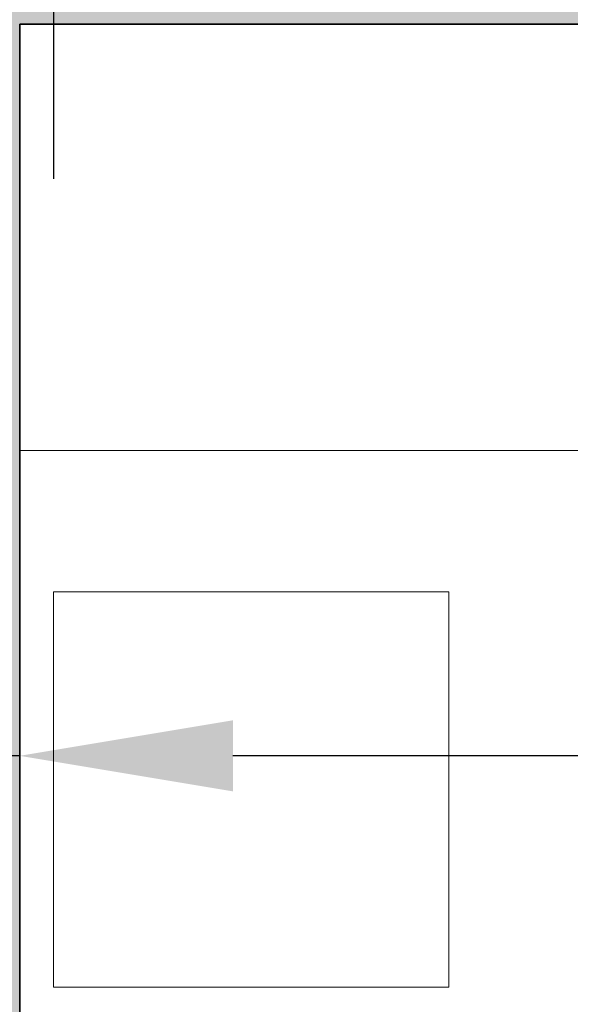
# Model space of a CAD drawing. Units: inches. Extents: x 2083 to 3317, y 1141 to 2115.
# Tile 12 of 256: x 2236 to 2267, y 1361 to 1417. Entities that reach past the tile are written whole.
import ezdxf

# ---------------------------------------------------------------- set-up
doc = ezdxf.new("R2010")
doc.units = ezdxf.units.IN
for name, color, linetype, lineweight in [('A-ANNO-DIMS', 2, 'Continuous', 18), ('A-FLOR-CASE', 8, 'Continuous', 18), ('A-FURN', 8, 'Continuous', 18), ('A-WALL', 7, 'Continuous', 35)]:
    doc.layers.add(name, color=color, linetype=linetype, lineweight=lineweight)
doc.layers.add('A-WALL-PATT', color=251, linetype='Continuous', lineweight=13, true_color=0x636466)
doc.styles.get("Standard").update_dxf_attribs({"font": 'arial.ttf'})
doc.dimstyles.new('ISO-25', dxfattribs={"dimtxt": 12, "dimasz": 12, "dimexe": 1.25, "dimexo": 0.625, "dimtad": 1, "dimlunit": 3, "dimtxsty": 'Standard', "dimcen": 2.5, "dimadec": 0, "dimazin": 0, "dimtfac": 1, "dimtmove": 0, "dimatfit": 3, "dimfxl": 1, "dimarcsym": 0})

# ---------------------------------------------------------------- blocks, each defined once
blk = doc.blocks.new('CASEWORK-96X24')
blk.add_line((0, 96), (0, 0))
blk = doc.blocks.new('NIGHTSTAND-COMPACT')
blk.add_lwpolyline([(22.254, 22.255), (22.254, 0), (0, 0), (0, 22.255)], close=True)
blk = doc.blocks.new('*D22')
at = {"layer": 'A-ANNO-DIMS', "color": 0, "lineweight": -2, "transparency": 16777216}
for p, q in [((2235.96, 1362.739), (2235.96, 1376.309)), ((2322.26, 1362.739), (2322.26, 1376.309)), ((2235.96, 1375.059), (2083.007, 1375.059)), ((2310.26, 1375.059), (2247.96, 1375.059))]:
    blk.add_line(p, q, dxfattribs=at)
at = {"layer": 'A-ANNO-DIMS', "color": 0, "transparency": 16777216}
for points in [[(2247.96, 1377.059), (2247.96, 1373.059), (2235.96, 1375.059)], [(2310.26, 1377.059), (2310.26, 1373.059), (2322.26, 1375.059)]]:
    blk.add_solid(points, dxfattribs=at)
at = {"layer": 'Defpoints', "color": 0, "transparency": 16777216}
for p in [(2235.96, 1375.059), (2235.96, 1362.114), (2322.26, 1362.114)]:
    blk.add_point(p, dxfattribs=at)
at = {"layer": 'A-ANNO-DIMS', "color": 0, "transparency": 16777216, "insert": (2153.483, 1381.889), "char_height": 12, "attachment_point": 5}
blk.add_mtext('BED 7\'-2 1/2" TYP.', dxfattribs=at)
blk = doc.blocks.new('*D30')
at = {"layer": 'A-ANNO-DIMS', "color": 0, "lineweight": -2, "transparency": 16777216}
for p, q in [((2240.018, 1445.274), (2240.018, 1448.046)), ((2254.329, 1445.274), (2254.329, 1448.046)), ((2228.018, 1446.796), (2216.018, 1446.796)), ((2240.018, 1446.796), (2254.329, 1446.796)), ((2266.329, 1446.796), (2413.765, 1446.796))]:
    blk.add_line(p, q, dxfattribs=at)
at = {"layer": 'A-ANNO-DIMS', "color": 0, "transparency": 16777216}
for points in [[(2228.018, 1448.796), (2228.018, 1444.796), (2240.018, 1446.796)], [(2266.329, 1448.796), (2266.329, 1444.796), (2254.329, 1446.796)]]:
    blk.add_solid(points, dxfattribs=at)
at = {"layer": 'Defpoints', "color": 0, "transparency": 16777216}
for p in [(2254.329, 1446.796), (2240.018, 1444.649), (2254.329, 1444.649)]:
    blk.add_point(p, dxfattribs=at)
at = {"layer": 'A-ANNO-DIMS', "color": 0, "transparency": 16777216, "insert": (2346.047, 1453.625), "char_height": 12, "attachment_point": 5}
blk.add_mtext('WC 1\'-2 1/2" TYP.', dxfattribs=at)
blk = doc.blocks.new('*D31')
at = {"layer": 'A-ANNO-DIMS', "color": 0, "lineweight": -2, "transparency": 16777216}
for p, q in [((2237.871, 1456.649), (2237.871, 1541.915)), ((2239.393, 1444.649), (2236.621, 1444.649)), ((2237.871, 1431.548), (2237.871, 1444.649)), ((2239.393, 1431.548), (2236.621, 1431.548)), ((2237.871, 1419.548), (2237.871, 1407.548))]:
    blk.add_line(p, q, dxfattribs=at)
at = {"layer": 'A-ANNO-DIMS', "color": 0, "transparency": 16777216}
for points in [[(2235.871, 1456.649), (2239.871, 1456.649), (2237.871, 1444.649)], [(2235.871, 1419.548), (2239.871, 1419.548), (2237.871, 1431.548)]]:
    blk.add_solid(points, dxfattribs=at)
at = {"layer": 'Defpoints', "color": 0, "transparency": 16777216}
for p in [(2237.871, 1444.649), (2240.018, 1444.649), (2240.018, 1431.548)]:
    blk.add_point(p, dxfattribs=at)
at = {"layer": 'A-ANNO-DIMS', "color": 0, "transparency": 16777216, "insert": (2231.217, 1505.282), "char_height": 12, "attachment_point": 5, "rotation": 90}
blk.add_mtext('1\'-1" TYP.', dxfattribs=at)

msp = doc.modelspace()

# ---------------------------------------------------------------- hatches: boundary and pattern name
at = {"layer": 'A-WALL-PATT'}
h = msp.add_hatch(color=256, dxfattribs=at)
h.dxf.hatch_style = 1
h.paths.add_polyline_path([(3126.96, 2020.761), (2748.96, 2020.761), (2604.96, 2020.761), (2226.96, 2020.761), (2226.96, 1702.761), (2466.96, 1702.761), (2466.96, 1582.761), (2418.96, 1582.761), (2418.96, 1477.761), (2226.96, 1477.761), (2226.96, 1263.261), (2544.96, 1263.261), (2544.96, 1411.761), (2604.96, 1411.761), (2685.96, 1411.761), (2685.96, 1420.761), (2604.96, 1420.761), (2604.96, 1573.761), (2604.96, 1702.761), (2604.96, 2011.761), (2748.96, 2011.761), (2748.96, 1702.761), (2862.96, 1702.761), (2862.96, 1621.761), (2871.96, 1621.761), (2871.96, 1702.761), (2883.96, 1702.761), (2883.96, 1706.939, -0.026459), (2883.96, 1711.761), (2757.96, 1711.761), (2757.96, 1807.761), (2787.96, 1807.761), (2787.96, 1812.261), (2757.96, 1812.261), (2757.96, 2011.761), (2877.96, 2011.761), (2877.96, 1812.261), (2847.96, 1812.261), (2847.96, 1807.761), (2889.836, 1807.761), (2889.836, 1812.261), (2882.46, 1812.261), (2882.46, 2011.761), (3117.96, 2011.761), (3117.96, 1812.261), (2937.836, 1812.261), (2937.836, 1807.761), (2995.71, 1807.761), (2995.71, 1796.118), (3000.21, 1796.118), (3000.21, 1807.761), (3117.96, 1807.761), (3117.96, 1711.761), (3000.21, 1711.761), (3000.21, 1760.118), (2998.573, 1760.118, -0.020711), (2995.71, 1760.118), (2995.71, 1711.761), (2931.96, 1711.761), (2931.96, 1702.761), (3126.96, 1702.761)])
h.paths.add_polyline_path([(2471.46, 2011.761), (2471.46, 1810.011), (2462.717, 1810.011), (2462.717, 1805.511), (2505.96, 1805.511), (2505.96, 1810.011), (2475.96, 1810.011), (2475.96, 2011.761), (2595.96, 2011.761), (2595.96, 1810.011), (2565.96, 1810.011), (2565.96, 1805.511), (2595.96, 1805.511), (2595.96, 1711.761), (2235.96, 1711.761), (2235.96, 1805.511), (2353.71, 1805.511), (2353.71, 1796.054), (2358.21, 1796.054), (2358.21, 1805.511), (2414.717, 1805.511), (2414.717, 1810.011), (2235.96, 1810.011), (2235.96, 2011.761)], flags=16)
h.paths.add_polyline_path([(2270.205, 1994.61), (2270.205, 1970.61), (2246.205, 1970.61), (2246.205, 1994.61)], flags=0)
edge = h.paths.add_edge_path(flags=0)
edge.add_ellipse((2332.027, 1899.798), major_axis=(-3.043, 3.043), ratio=0.168252, start_angle=-161.3322, end_angle=-156.3071, ccw=False)
edge.add_ellipse((2333.082, 1898.744), major_axis=(-1.055, 1.055), ratio=0.453532, start_angle=-123.371, end_angle=-94.1591)
edge = h.paths.add_edge_path(flags=0)
edge.add_ellipse((2332.027, 1968.876), major_axis=(3.043, 3.043), ratio=0.168252, start_angle=18.6678, end_angle=23.6929)
edge.add_spline(control_points=[(2332.926, 1970.691), (2332.227, 1970.336), (2330.894, 1969.659), (2328.413, 1970.932), (2327.204, 1967.749), (2324.71, 1969.956), (2322.533, 1967.012), (2320.013, 1971.296), (2317.68, 1968.158), (2316.041, 1967.102), (2315.427, 1966.81)], knot_values=[0, 0, 0, 0, 2.267059, 4.324559, 6.685584, 8.878641, 11.121502, 14.300359, 17.755284, 19.732645, 19.732645, 19.732645, 19.732645], degree=3, periodic=0)
edge.add_ellipse((2332.027, 1968.876), major_axis=(3.043, 3.043), ratio=0.168252, start_angle=18.6678, end_angle=23.6929, ccw=False)
edge.add_ellipse((2333.082, 1969.931), major_axis=(1.055, 1.055), ratio=0.453532, start_angle=56.629, end_angle=85.8409, ccw=False)
edge = h.paths.add_edge_path(flags=0)
edge.add_spline(control_points=[(2296.428, 1967.988), (2293.628, 1965.336), (2287.704, 1959.727), (2299.744, 1949.996), (2294.533, 1935.669), (2290.573, 1920.604), (2293.394, 1909.974), (2296.185, 1904.967)], knot_values=[0.099185, 0.099185, 0.099185, 0.099185, 0.345301, 0.619822, 0.982653, 1.386093, 1.810555, 1.810555, 1.810555, 1.810555], degree=3, periodic=0)
edge.add_spline(control_points=[(2296.185, 1904.967), (2297.384, 1902.619), (2298.001, 1901.949), (2298.553, 1901.468)], knot_values=[0.006246, 0.006246, 0.006246, 0.006246, 0.055476, 0.055476, 0.055476, 0.055476], degree=3, periodic=0)
edge.add_spline(control_points=[(2298.553, 1901.468), (2297.259, 1900.923), (2295.225, 1900.232), (2293.06, 1900.614), (2292.101, 1900.788), (2292.09, 1900.791)], knot_values=[0.312835, 0.312835, 0.312835, 0.312835, 0.40178, 0.474987, 0.475903, 0.475903, 0.475903, 0.475903], degree=3, periodic=0)
edge.add_arc((2292.794, 1904.664), 3.937, 215.4209, 259.6982, ccw=False)
edge.add_spline(control_points=[(2289.585, 1902.382), (2289.477, 1902.535), (2289.368, 1902.688), (2289.261, 1902.841)], knot_values=[0.102872, 0.102872, 0.102872, 0.102872, 0.116896, 0.116896, 0.116896, 0.116896], degree=3, periodic=0)
edge.add_spline(control_points=[(2289.261, 1902.841), (2288.687, 1902.55), (2287.64, 1902.02), (2285.881, 1901.874), (2283.853, 1901.504), (2281.72, 1899.711), (2278.467, 1899.493), (2276.157, 1901.883), (2272.259, 1899.804), (2267.778, 1901.843), (2262.244, 1900.184), (2257.415, 1901.782), (2254.318, 1900.726), (2253.178, 1900.337)], knot_values=[0, 0, 0, 0, 1.907977, 3.477176, 5.261074, 7.972851, 11.680248, 13.717921, 16.939592, 22.789562, 27.502503, 33.595215, 37.145618, 37.145618, 37.145618, 37.145618], degree=3, periodic=0)
edge.add_line((2253.178, 1900.337), (2250.244, 1902.841))
edge.add_line((2250.244, 1902.841), (2250.244, 1965.833))
edge.add_line((2250.244, 1965.833), (2253.178, 1968.337))
edge.add_spline(control_points=[(2253.178, 1968.337), (2254.318, 1967.948), (2257.415, 1966.892), (2262.244, 1968.49), (2267.778, 1966.831), (2271.527, 1968.537), (2273.876, 1967.828), (2274.207, 1967.728)], knot_values=[0, 0, 0, 0, 0.09018, 0.244935, 0.364644, 0.513233, 0.537855, 0.537855, 0.537855, 0.537855], degree=3, periodic=0)
edge.add_arc((2274.353, 1963.793), 3.937, 72.0511, 92.1279, ccw=False)
edge.add_arc((2281.297, 1985.23), 18.596, 252.0511, 288.5657)
edge.add_arc((2292.317, 1956.029), 12.646, 71.0268, 113.7782, ccw=False)
edge = h.paths.add_edge_path(flags=0)
edge.add_spline(control_points=[(2274.899, 1951.856), (2275.066, 1951.617), (2275.233, 1951.377), (2275.398, 1951.136)], knot_values=[1.409916, 1.409916, 1.409916, 1.409916, 1.43159, 1.43159, 1.43159, 1.43159], degree=3, periodic=0)
edge.add_spline(control_points=[(2275.398, 1951.136), (2275.792, 1950.562), (2276.179, 1949.984), (2276.546, 1949.397)], knot_values=[1.358238, 1.358238, 1.358238, 1.358238, 1.409916, 1.409916, 1.409916, 1.409916], degree=3, periodic=0)
edge.add_line((2276.546, 1949.397), (2277.437, 1947.862))
edge.add_spline(control_points=[(2277.437, 1947.862), (2276.304, 1945.673), (2274.64, 1942.427), (2274.632, 1938.094), (2272.799, 1930.852), (2274.356, 1943.897), (2275.948, 1947.923), (2276.546, 1949.397)], knot_values=[0.005632, 0.005632, 0.005632, 0.005632, 0.186014, 0.266002, 0.357087, 0.59639, 0.739732, 0.739732, 0.739732, 0.739732], degree=3, periodic=0)
edge.add_spline(control_points=[(2276.546, 1949.397), (2276.179, 1949.984), (2275.792, 1950.562), (2275.398, 1951.136)], knot_values=[1.358238, 1.358238, 1.358238, 1.358238, 1.409916, 1.409916, 1.409916, 1.409916], degree=3, periodic=0)
edge.add_spline(control_points=[(2275.398, 1951.136), (2274.943, 1950.08), (2274.208, 1948.025), (2273.935, 1944.851), (2272.469, 1937.627), (2273.466, 1945.696), (2274.701, 1951.059), (2274.899, 1951.856)], knot_values=[0.104364, 0.104364, 0.104364, 0.104364, 0.189636, 0.269624, 0.36071, 0.600013, 0.644622, 0.644622, 0.644622, 0.644622], degree=3, periodic=0)
h.paths.add_polyline_path([(2269.168, 1963.128, -0.357527), (2268.171, 1960.976, -0.092561), (2268.171, 1939.436, -0.357527), (2269.168, 1937.285, -0.357527), (2267.016, 1938.282, -0.164785), (2254.686, 1938.282, -0.357527), (2252.534, 1937.285, -0.357527), (2253.531, 1939.436, -0.092561), (2253.531, 1960.976, -0.357527), (2252.534, 1963.128, -0.357527), (2254.686, 1962.131, -0.164785), (2267.016, 1962.131, -0.357527)], flags=0)
h.paths.add_polyline_path([(2248.874, 1967.802), (2248.874, 1957.028), (2249.458, 1957.028), (2249.458, 1911.647), (2248.874, 1911.647), (2248.874, 1900.873), (2246.512, 1900.873, 0.197327), (2244.15, 1902.457), (2244.15, 1966.218, 0.197327), (2246.512, 1967.802)], flags=0)
h.paths.add_polyline_path([(2269.168, 1931.389, -0.357527), (2268.171, 1929.238, -0.092561), (2268.171, 1907.698, -0.357527), (2269.168, 1905.547, -0.357527), (2267.016, 1906.544, -0.164785), (2254.686, 1906.544, -0.357527), (2252.534, 1905.547, -0.357527), (2253.531, 1907.698, -0.092561), (2253.531, 1929.238, -0.357527), (2252.534, 1931.389, -0.357527), (2254.686, 1930.392, -0.164785), (2267.016, 1930.392, -0.357527)], flags=0)
edge = h.paths.add_edge_path(flags=0)
edge.add_spline(control_points=[(2276.197, 1906.724), (2276.168, 1909.029), (2276.114, 1913.372), (2270.598, 1924.925), (2273.905, 1919.013), (2275.922, 1916.262), (2275.475, 1912.402), (2277.258, 1910.381), (2276.696, 1908.225), (2276.646, 1906.813), (2276.618, 1906.008)], knot_values=[0, 0, 0, 0, 8.61026, 16.221274, 18.843057, 23.804898, 27.440828, 29.356102, 31.203478, 33.650687, 33.650687, 33.650687, 33.650687], degree=3, periodic=0)
edge.add_spline(control_points=[(2276.618, 1906.008), (2276.623, 1905.624), (2276.498, 1904.629), (2275.442, 1903.855), (2274.937, 1903.08), (2274.859, 1902.841)], knot_values=[0.156488, 0.156488, 0.156488, 0.156488, 0.184398, 0.231376, 0.250598, 0.250598, 0.250598, 0.250598], degree=3, periodic=0)
edge.add_line((2274.859, 1902.841), (2276.506, 1902.841))
edge.add_spline(control_points=[(2276.506, 1902.841), (2276.788, 1903.085), (2277.665, 1904.125), (2278.25, 1904.341), (2277.654, 1908.527), (2278.156, 1906.228), (2278.1, 1905.286), (2278.847, 1904.069), (2277.857, 1903.415), (2277.874, 1902.991), (2277.904, 1902.841)], knot_values=[0.059574, 0.059574, 0.059574, 0.059574, 0.080753, 0.103741, 0.16972, 0.176036, 0.207137, 0.240474, 0.262341, 0.27366, 0.27366, 0.27366, 0.27366], degree=3, periodic=0)
edge.add_line((2277.904, 1902.841), (2280.03, 1902.841))
edge.add_spline(control_points=[(2280.03, 1902.841), (2279.888, 1903.088), (2279.499, 1903.982), (2280.152, 1905.939), (2278.104, 1909.658), (2279.762, 1907.185), (2280.328, 1904.875), (2280.485, 1903.49), (2281.463, 1903.249), (2281.758, 1902.936), (2281.834, 1902.841)], knot_values=[0.013856, 0.013856, 0.013856, 0.013856, 0.034874, 0.088867, 0.107879, 0.126738, 0.158714, 0.193757, 0.217487, 0.226722, 0.226722, 0.226722, 0.226722], degree=3, periodic=0)
edge.add_spline(control_points=[(2281.834, 1902.841), (2281.788, 1902.827), (2281.647, 1902.783), (2281.396, 1902.859), (2281.088, 1902.985), (2280.721, 1903.061), (2280.333, 1903.026), (2280.125, 1902.899), (2280.03, 1902.841)], knot_values=[0, 0, 0, 0, 0.14413, 0.435517, 0.749276, 1.153046, 1.548371, 1.878348, 1.878348, 1.878348, 1.878348], degree=3, periodic=0)
edge.add_line((2280.03, 1902.841), (2277.904, 1902.841))
edge.add_spline(control_points=[(2277.904, 1902.841), (2277.893, 1902.796), (2277.865, 1902.68), (2277.607, 1902.687), (2277.274, 1902.801), (2276.838, 1902.62), (2276.584, 1902.789), (2276.506, 1902.841)], knot_values=[0, 0, 0, 0, 0.127189, 0.326199, 0.628009, 1.24357, 1.515331, 1.515331, 1.515331, 1.515331], degree=3, periodic=0)
edge.add_line((2276.506, 1902.841), (2274.859, 1902.841))
edge.add_spline(control_points=[(2274.859, 1902.841), (2274.814, 1902.899), (2274.725, 1903.013), (2274.493, 1903.119), (2274.244, 1902.961), (2273.937, 1903.185), (2273.614, 1902.983), (2273.408, 1902.883), (2273.322, 1902.841)], knot_values=[0, 0, 0, 0, 0.21843, 0.436957, 0.687977, 0.990379, 1.398396, 1.69185, 1.69185, 1.69185, 1.69185], degree=3, periodic=0)
edge.add_spline(control_points=[(2273.322, 1902.841), (2273.617, 1903.446), (2274.274, 1904.538), (2276.027, 1904.574), (2276.207, 1906.584), (2276.197, 1906.724)], knot_values=[0.012227, 0.012227, 0.012227, 0.012227, 0.059472, 0.106218, 0.134458, 0.134458, 0.134458, 0.134458], degree=3, periodic=0)
h.paths.add_polyline_path([(2270.776, 1897.79), (2270.776, 1873.79), (2246.776, 1873.79), (2246.776, 1897.79)], flags=0)
h.paths.add_polyline_path([(2353.71, 1760.005), (2353.71, 1760.054), (2358.21, 1760.054, -0.033729)], flags=0)
h.paths.add_polyline_path([(2321.819, 1737.529), (2341.995, 1737.529, -0.414214), (2343.203, 1736.321), (2343.203, 1721.021, -0.414214), (2341.995, 1719.813), (2321.819, 1719.813, -0.414214), (2320.611, 1721.021), (2320.611, 1736.321, -0.414214)], flags=0)
h.paths.add_polyline_path([(2324.235, 1736.321), (2339.579, 1736.321, -0.414214), (2341.995, 1733.905), (2341.995, 1725.45, -0.414214), (2339.579, 1723.034), (2333.681, 1723.034), (2333.845, 1722.045, -0.870646), (2335.425, 1721.826, -0.767327), (2333.923, 1721.423), (2331.291, 1721.423, -0.767327), (2329.788, 1721.826, -0.870646), (2331.368, 1722.045), (2331.533, 1723.034), (2324.235, 1723.034, -0.414214), (2321.819, 1725.45), (2321.819, 1733.905, -0.414214)], flags=0)
h.paths.add_polyline_path([(2570.484, 1928.615), (2589.684, 1928.615), (2590.169, 1928.615), (2590.169, 1904.993), (2570.484, 1904.993)], flags=0)
h.paths.add_polyline_path([(2574.447, 1927.264, -1), (2572.829, 1927.264, -1)], flags=0)
h.paths.add_polyline_path([(2573.09, 1926.941), (2573.925, 1927.776), (2574.148, 1927.553), (2573.313, 1926.718)], flags=0)
h.paths.add_polyline_path([(2578.779, 1919.73, -1), (2571.592, 1919.73, -1)], flags=0)
h.paths.add_polyline_path([(2578.385, 1919.73, -1), (2571.985, 1919.73, -1)], flags=0)
h.paths.add_polyline_path([(2331.596, 1729.476, -1), (2333.618, 1729.476, -1)], flags=0)
h.paths.add_polyline_path([(2578.034, 1927.264, -1), (2576.416, 1927.264, -1)], flags=0)
h.paths.add_polyline_path([(2576.689, 1927.531), (2576.912, 1927.754), (2577.747, 1926.919), (2577.524, 1926.696)], flags=0)
h.paths.add_polyline_path([(2578.139, 1909.86, -1), (2572.232, 1909.86, -1)], flags=0)
h.paths.add_polyline_path([(2577.745, 1909.86, -1), (2572.625, 1909.86, -1)], flags=0)
h.paths.add_polyline_path([(2583.798, 1927.264, -1), (2582.179, 1927.264, -1)], flags=0)
h.paths.add_polyline_path([(2582.719, 1927.754), (2583.554, 1926.919), (2583.331, 1926.696), (2582.496, 1927.531)], flags=0)
h.paths.add_polyline_path([(2582.496, 1927.531), (2582.719, 1927.754), (2583.554, 1926.919), (2583.331, 1926.696)], flags=0)
h.paths.add_polyline_path([(2587.739, 1920.53, -1), (2581.832, 1920.53, -1)], flags=0)
h.paths.add_polyline_path([(2587.345, 1920.53, -1), (2582.225, 1920.53, -1)], flags=0)
h.paths.add_polyline_path([(2587.385, 1927.264, -1), (2585.766, 1927.264, -1)], flags=0)
h.paths.add_polyline_path([(2586.082, 1926.98), (2586.917, 1927.815), (2587.14, 1927.593), (2586.305, 1926.758)], flags=0)
h.paths.add_polyline_path([(2588.379, 1910.66, -1), (2581.192, 1910.66, -1)], flags=0)
h.paths.add_polyline_path([(2587.985, 1910.66, -1), (2581.585, 1910.66, -1)], flags=0)
h.paths.add_polyline_path([(2417.168, 1729.478), (2437.344, 1729.478, -0.414214), (2438.552, 1728.27), (2438.552, 1712.969, -0.414214), (2437.344, 1711.761), (2417.168, 1711.761, -0.414214), (2415.96, 1712.969), (2415.96, 1728.27, -0.414214)], flags=0)
h.paths.add_polyline_path([(2419.584, 1728.27), (2434.928, 1728.27, -0.414214), (2437.344, 1725.854), (2437.344, 1717.398, -0.414214), (2434.928, 1714.983), (2429.029, 1714.983), (2429.194, 1713.994, -0.870646), (2430.774, 1713.775, -0.767327), (2429.271, 1713.372), (2426.64, 1713.372, -0.767327), (2425.137, 1713.775, -0.870646), (2426.717, 1713.994), (2426.882, 1714.983), (2419.584, 1714.983, -0.414214), (2417.168, 1717.398), (2417.168, 1725.854, -0.414214)], flags=0)
h.paths.add_polyline_path([(2419.584, 1728.27), (2434.928, 1728.27, -0.414214), (2437.344, 1725.854), (2437.344, 1717.398, -0.414214), (2434.928, 1714.983), (2429.029, 1714.983), (2428.358, 1719.009), (2427.553, 1719.009), (2426.882, 1714.983), (2419.584, 1714.983, -0.414214), (2417.168, 1717.398), (2417.168, 1725.854, -0.414214)], flags=0)
h.paths.add_polyline_path([(2426.944, 1721.425, -1), (2428.967, 1721.425, -1)], flags=0)
h.paths.add_polyline_path([(2475.96, 1702.761), (2595.96, 1702.761), (2595.96, 1582.761), (2475.96, 1582.761)], flags=16)
h.paths.add_polyline_path([(2427.96, 1573.761), (2595.96, 1573.761), (2595.96, 1468.761), (2595.96, 1420.761), (2384.46, 1420.761), (2384.46, 1468.761), (2427.96, 1468.761)], flags=16)
h.paths.add_polyline_path([(2379.96, 1468.761), (2379.96, 1420.761), (2235.96, 1420.761), (2235.96, 1468.761)], flags=16)
h.paths.add_polyline_path([(2317.816, 1466.696), (2337.992, 1466.696, -0.414214), (2339.2, 1465.488), (2339.2, 1450.187, -0.414214), (2337.992, 1448.979), (2317.816, 1448.979, -0.414214), (2316.608, 1450.187), (2316.608, 1465.488, -0.414214)], flags=0)
h.paths.add_polyline_path([(2320.232, 1465.488), (2335.576, 1465.488, -0.414214), (2337.992, 1463.072), (2337.992, 1454.616, -0.414214), (2335.576, 1452.2), (2329.677, 1452.2), (2329.842, 1451.212, -0.870646), (2331.422, 1450.992, -0.767327), (2329.92, 1450.59), (2327.288, 1450.59, -0.767327), (2325.785, 1450.992, -0.870646), (2327.365, 1451.212), (2327.53, 1452.2), (2320.232, 1452.2, -0.414214), (2317.816, 1454.616), (2317.816, 1463.072, -0.414214)], flags=0)
h.paths.add_polyline_path([(2320.232, 1465.488), (2335.576, 1465.488, -0.414214), (2337.992, 1463.072), (2337.992, 1454.616, -0.414214), (2335.576, 1452.2), (2329.677, 1452.2), (2329.006, 1456.227), (2328.201, 1456.227), (2327.53, 1452.2), (2320.232, 1452.2, -0.414214), (2317.816, 1454.616), (2317.816, 1463.072, -0.414214)], flags=0)
h.paths.add_polyline_path([(2327.593, 1458.643, -1), (2329.615, 1458.643, -1)], flags=0)
h.paths.add_polyline_path([(2244.412, 1433.34), (2241.921, 1433.34, -0.414214), (2240.018, 1435.244), (2240.018, 1440.953, -0.414211), (2241.921, 1442.856), (2244.412, 1442.856, -1.976472)], flags=0)
h.paths.add_polyline_path([(2245.357, 1434.398, -0.414214), (2245.357, 1441.799, -2.144098)], flags=0)
h.paths.add_polyline_path([(2535.96, 1416.261), (2535.96, 1272.261), (2235.96, 1272.261), (2235.96, 1416.261)], flags=16)
h.paths.add_polyline_path([(2260.12, 1384.293), (2260.12, 1362.039), (2237.865, 1362.039), (2237.865, 1384.293)], flags=0)
edge = h.paths.add_edge_path(flags=0)
edge.add_line((2318.252, 1362.093), (2318.146, 1362.001))
edge.add_ellipse((2317.445, 1360.431), major_axis=(2.822, 2.822), ratio=0.168252, start_angle=18.6678, end_angle=20.9481, ccw=False)
edge.add_ellipse((2318.423, 1361.409), major_axis=(0.978, 0.978), ratio=0.453532, start_angle=56.629, end_angle=70.2262, ccw=False)
edge = h.paths.add_edge_path(flags=0)
edge.add_line((2319.107, 1295.571), (2319.015, 1295.677))
edge.add_ellipse((2317.445, 1296.378), major_axis=(-2.822, 2.822), ratio=0.168252, start_angle=-161.3322, end_angle=-159.0519, ccw=False)
edge.add_ellipse((2318.423, 1295.4), major_axis=(-0.978, 0.978), ratio=0.453532, start_angle=-123.371, end_angle=-109.7738)
edge = h.paths.add_edge_path(flags=0)
edge.add_spline(control_points=[(2284.21, 1301.17), (2284.581, 1300.445), (2284.891, 1299.892), (2285.16, 1299.461)], knot_values=[0.039066, 0.039066, 0.039066, 0.039066, 0.055476, 0.055476, 0.055476, 0.055476], degree=3, periodic=0)
edge.add_line((2285.16, 1299.461), (2284.21, 1301.17))
edge = h.paths.add_edge_path(flags=0)
edge.add_line((2280.412, 1297.298), (2283.37, 1297.036))
edge.add_line((2283.37, 1297.036), (2286.406, 1297.926))
edge.add_spline(control_points=[(2286.406, 1297.926), (2285.305, 1297.463), (2284.345, 1297.129), (2283.37, 1297.036)], knot_values=[0.394369, 0.394369, 0.394369, 0.394369, 0.475903, 0.475903, 0.475903, 0.475903], degree=3, periodic=0)
edge.add_spline(control_points=[(2283.37, 1297.036), (2283.281, 1297.028), (2282.316, 1296.957), (2281.313, 1297.134), (2280.423, 1297.296), (2280.412, 1297.298)], knot_values=[0.312835, 0.312835, 0.312835, 0.312835, 0.320246, 0.393453, 0.394369, 0.394369, 0.394369, 0.394369], degree=3, periodic=0)
edge = h.paths.add_edge_path(flags=0)
edge.add_line((2284.436, 1359.607), (2280.446, 1355.328))
edge.add_line((2280.446, 1355.328), (2279.58, 1351.018))
edge.add_line((2279.58, 1351.018), (2282.413, 1346.58))
edge.add_spline(control_points=[(2282.413, 1346.58), (2283.153, 1345.589), (2284.253, 1344.029), (2284.801, 1342.387), (2284.935, 1341.806)], knot_values=[1.240098, 1.240098, 1.240098, 1.240098, 1.332892, 1.382712, 1.382712, 1.382712, 1.382712], degree=3, periodic=0)
edge.add_spline(control_points=[(2284.935, 1341.806), (2285.319, 1340.141), (2285.233, 1338.409), (2284.91, 1336.654)], knot_values=[1.097484, 1.097484, 1.097484, 1.097484, 1.240098, 1.240098, 1.240098, 1.240098], degree=3, periodic=0)
edge.add_spline(control_points=[(2284.91, 1336.654), (2284.587, 1334.899), (2284.027, 1333.12), (2283.463, 1331.361)], knot_values=[0.95487, 0.95487, 0.95487, 0.95487, 1.097484, 1.097484, 1.097484, 1.097484], degree=3, periodic=0)
edge.add_line((2283.463, 1331.361), (2281.89, 1326.153))
edge.add_line((2281.89, 1326.153), (2280.756, 1321.056))
edge.add_line((2280.756, 1321.056), (2280.299, 1316.002))
edge.add_line((2280.299, 1316.002), (2280.716, 1310.95))
edge.add_line((2280.716, 1310.95), (2282.028, 1305.972))
edge.add_line((2282.028, 1305.972), (2284.21, 1301.17))
edge.add_spline(control_points=[(2284.21, 1301.17), (2283.341, 1302.73), (2282.612, 1304.336), (2282.028, 1305.972)], knot_values=[0.099185, 0.099185, 0.099185, 0.099185, 0.241799, 0.241799, 0.241799, 0.241799], degree=3, periodic=0)
edge.add_spline(control_points=[(2282.028, 1305.972), (2281.444, 1307.608), (2281.005, 1309.273), (2280.716, 1310.95)], knot_values=[0.241799, 0.241799, 0.241799, 0.241799, 0.384413, 0.384413, 0.384413, 0.384413], degree=3, periodic=0)
edge.add_spline(control_points=[(2280.716, 1310.95), (2280.433, 1312.588), (2280.289, 1314.277), (2280.299, 1315.962), (2280.299, 1316.002)], knot_values=[0.384413, 0.384413, 0.384413, 0.384413, 0.523647, 0.527028, 0.527028, 0.527028, 0.527028], degree=3, periodic=0)
edge.add_spline(control_points=[(2280.299, 1316.002), (2280.312, 1317.687), (2280.478, 1319.368), (2280.756, 1321.056)], knot_values=[0.527028, 0.527028, 0.527028, 0.527028, 0.669642, 0.669642, 0.669642, 0.669642], degree=3, periodic=0)
edge.add_spline(control_points=[(2280.756, 1321.056), (2281.035, 1322.744), (2281.426, 1324.44), (2281.89, 1326.153)], knot_values=[0.669642, 0.669642, 0.669642, 0.669642, 0.812256, 0.812256, 0.812256, 0.812256], degree=3, periodic=0)
edge.add_spline(control_points=[(2281.89, 1326.153), (2282.264, 1327.533), (2282.788, 1329.262), (2283.353, 1331.018), (2283.463, 1331.361)], knot_values=[0.812256, 0.812256, 0.812256, 0.812256, 0.927087, 0.95487, 0.95487, 0.95487, 0.95487], degree=3, periodic=0)
edge.add_line((2283.463, 1331.361), (2284.91, 1336.654))
edge.add_line((2284.91, 1336.654), (2284.935, 1341.806))
edge.add_line((2284.935, 1341.806), (2282.413, 1346.58))
edge.add_spline(control_points=[(2282.413, 1346.58), (2281.275, 1348.104), (2280.078, 1349.57), (2279.58, 1351.018)], knot_values=[1.382712, 1.382712, 1.382712, 1.382712, 1.525326, 1.525326, 1.525326, 1.525326], degree=3, periodic=0)
edge.add_spline(control_points=[(2279.58, 1351.018), (2279.443, 1351.415), (2279.136, 1352.857), (2279.735, 1354.29), (2280.446, 1355.328)], knot_values=[1.525326, 1.525326, 1.525326, 1.525326, 1.564439, 1.667941, 1.667941, 1.667941, 1.667941], degree=3, periodic=0)
edge.add_spline(control_points=[(2280.446, 1355.328), (2281.426, 1356.758), (2282.931, 1358.183), (2284.436, 1359.607)], knot_values=[1.667941, 1.667941, 1.667941, 1.667941, 1.810555, 1.810555, 1.810555, 1.810555], degree=3, periodic=0)
edge.add_arc((2280.623, 1348.518), 11.726, 71.0268, 113.7782)
edge.add_arc((2270.405, 1375.595), 17.244, 252.0511, 288.5657, ccw=False)
edge.add_arc((2263.966, 1355.718), 3.651, 72.0511, 92.1279)
edge.add_arc((2263.966, 1355.718), 3.651, 92.1279, 177.9851)
edge.add_spline(control_points=[(2260.318, 1355.846), (2260.26, 1354.221), (2260.551, 1350.187), (2262.999, 1346.766), (2264.473, 1344.649)], knot_values=[1.43159, 1.43159, 1.43159, 1.43159, 1.564144, 1.770695, 1.770695, 1.770695, 1.770695], degree=3, periodic=0)
edge.add_line((2264.473, 1344.649), (2264.936, 1343.983))
edge.add_spline(control_points=[(2263.801, 1340.248), (2263.843, 1340.514), (2264.067, 1341.756), (2264.513, 1343.002), (2264.935, 1343.981)], knot_values=[0.53657, 0.53657, 0.53657, 0.53657, 0.559349, 0.644622, 0.644622, 0.644622, 0.644622], degree=3, periodic=0)
edge.add_spline(control_points=[(2264.935, 1343.981), (2265.118, 1343.715), (2265.299, 1343.448), (2265.477, 1343.179)], knot_values=[1.384077, 1.384077, 1.384077, 1.384077, 1.409916, 1.409916, 1.409916, 1.409916], degree=3, periodic=0)
edge.add_spline(control_points=[(2265.477, 1343.179), (2265.655, 1342.911), (2265.829, 1342.641), (2265.999, 1342.369)], knot_values=[1.358238, 1.358238, 1.358238, 1.358238, 1.384077, 1.384077, 1.384077, 1.384077], degree=3, periodic=0)
edge.add_line((2265.999, 1342.369), (2266.826, 1340.946))
edge.add_spline(control_points=[(2266.826, 1340.946), (2268.894, 1337.09), (2271.398, 1325.843), (2270.516, 1310.569), (2275.919, 1301.861), (2277.79, 1299.199)], knot_values=[0.116896, 0.116896, 0.116896, 0.116896, 0.472987, 1.050969, 1.313793, 1.313793, 1.313793, 1.313793], degree=3, periodic=0)
edge.add_spline(control_points=[(2277.79, 1299.199), (2277.839, 1299.128), (2277.889, 1299.057), (2277.94, 1298.987)], knot_values=[0.109884, 0.109884, 0.109884, 0.109884, 0.116896, 0.116896, 0.116896, 0.116896], degree=3, periodic=0)
edge.add_line((2277.94, 1298.987), (2277.789, 1299.199))
edge.add_spline(control_points=[(2277.789, 1299.199), (2277.257, 1298.929), (2276.286, 1298.438), (2275.039, 1298.334), (2274.383, 1298.239), (2274.215, 1298.209)], knot_values=[33.12187, 33.12187, 33.12187, 33.12187, 35.029056, 36.598255, 37.144827, 37.144827, 37.144827, 37.144827], degree=3, periodic=0)
edge.add_line((2274.215, 1298.209), (2273.073, 1297.893))
edge.add_spline(control_points=[(2273.073, 1297.893), (2272.323, 1297.58), (2271.039, 1296.511), (2269.248, 1296.226), (2268.423, 1296.375)], knot_values=[26.532584, 26.532584, 26.532584, 26.532584, 29.198919, 31.839101, 31.839101, 31.839101, 31.839101], degree=3, periodic=0)
edge.add_line((2268.423, 1296.375), (2263.879, 1297.458))
edge.add_spline(control_points=[(2263.879, 1297.458), (2263.556, 1297.359), (2261.86, 1296.839), (2260.239, 1297.282), (2258.933, 1297.516)], knot_values=[15.919551, 15.919551, 15.919551, 15.919551, 16.939592, 21.226067, 21.226067, 21.226067, 21.226067], degree=3, periodic=0)
edge.add_line((2258.933, 1297.516), (2254.055, 1297.329))
edge.add_spline(control_points=[(2254.055, 1297.329), (2253.756, 1297.296), (2252.114, 1297.165), (2250.462, 1297.544), (2249.13, 1297.668)], knot_values=[5.306517, 5.306517, 5.306517, 5.306517, 6.276435, 10.613034, 10.613034, 10.613034, 10.613034], degree=3, periodic=0)
edge.add_line((2249.13, 1297.668), (2244.332, 1296.878))
edge.add_line((2244.332, 1296.878), (2241.611, 1299.199))
edge.add_line((2241.611, 1299.199), (2241.611, 1357.609))
edge.add_line((2241.611, 1357.609), (2244.332, 1359.931))
edge.add_line((2244.332, 1359.931), (2252.729, 1359.543))
edge.add_spline(control_points=[(2252.729, 1359.543), (2252.871, 1359.546), (2253.306, 1359.548), (2253.74, 1359.514), (2254.032, 1359.482)], knot_values=[0.233291, 0.233291, 0.233291, 0.233291, 0.244935, 0.268927, 0.268927, 0.268927, 0.268927], degree=3, periodic=0)
edge.add_line((2254.032, 1359.482), (2259.587, 1359.416))
edge.add_spline(control_points=[(2259.587, 1359.416), (2260.677, 1359.629), (2262.073, 1359.897), (2263.524, 1359.459), (2263.83, 1359.366)], knot_values=[0.422516, 0.422516, 0.422516, 0.422516, 0.513233, 0.537855, 0.537855, 0.537855, 0.537855], degree=3, periodic=0)
edge.add_arc((2263.966, 1355.718), 3.651, 72.0511, 92.1279, ccw=False)
edge.add_arc((2270.405, 1375.595), 17.244, 252.0511, 288.5657)
edge.add_arc((2280.623, 1348.518), 11.726, 71.0268, 113.7782, ccw=False)
h.paths.add_polyline_path([(2240.341, 1359.435), (2240.341, 1349.444), (2240.882, 1349.444), (2240.882, 1307.365), (2240.341, 1307.365), (2240.341, 1297.374), (2238.15, 1297.374, 0.197327), (2235.96, 1298.843), (2235.96, 1357.966, 0.197327), (2238.15, 1359.435)], flags=0)
h.paths.add_polyline_path([(2259.158, 1355.101, -0.357527), (2258.233, 1353.106, -0.092561), (2258.233, 1333.133, -0.357527), (2259.158, 1331.138, -0.357527), (2257.163, 1332.062, -0.164785), (2245.729, 1332.062, -0.357527), (2243.735, 1331.138, -0.357527), (2244.659, 1333.133, -0.092561), (2244.659, 1353.106, -0.357527), (2243.735, 1355.101, -0.357527), (2245.729, 1354.176, -0.164785), (2257.163, 1354.176, -0.357527)], flags=0)
edge = h.paths.add_edge_path(flags=0)
edge.add_line((2265.999, 1342.369), (2266.826, 1340.946))
edge.add_line((2266.826, 1340.946), (2265.308, 1337.814))
edge.add_line((2265.308, 1337.814), (2264.358, 1334.653))
edge.add_line((2264.358, 1334.653), (2264.262, 1333.8))
edge.add_spline(control_points=[(2264.262, 1333.8), (2264.208, 1333.187), (2264.162, 1332.366), (2264.007, 1331.414), (2263.969, 1331.202)], knot_values=[0.464444, 0.464444, 0.464444, 0.464444, 0.516691, 0.531608, 0.531608, 0.531608, 0.531608], degree=3, periodic=0)
edge.add_spline(control_points=[(2263.969, 1331.202), (2263.775, 1330.119), (2263.424, 1328.791), (2263.257, 1328.531), (2263.234, 1328.515)], knot_values=[0.372682, 0.372682, 0.372682, 0.372682, 0.44885, 0.464444, 0.464444, 0.464444, 0.464444], degree=3, periodic=0)
edge.add_spline(control_points=[(2263.234, 1328.515), (2263.096, 1328.42), (2263.131, 1329.301), (2263.275, 1330.616)], knot_values=[0.280919, 0.280919, 0.280919, 0.280919, 0.372682, 0.372682, 0.372682, 0.372682], degree=3, periodic=0)
edge.add_spline(control_points=[(2263.275, 1330.616), (2263.419, 1331.93), (2263.672, 1333.677), (2263.97, 1335.315)], knot_values=[0.189157, 0.189157, 0.189157, 0.189157, 0.280919, 0.280919, 0.280919, 0.280919], degree=3, periodic=0)
edge.add_spline(control_points=[(2263.97, 1335.315), (2264.1, 1336.032), (2264.419, 1337.622), (2264.755, 1338.864), (2264.947, 1339.491)], knot_values=[0.097394, 0.097394, 0.097394, 0.097394, 0.137578, 0.189157, 0.189157, 0.189157, 0.189157], degree=3, periodic=0)
edge.add_spline(control_points=[(2264.947, 1339.491), (2265.29, 1340.606), (2265.644, 1341.494), (2265.999, 1342.369)], knot_values=[0.005632, 0.005632, 0.005632, 0.005632, 0.097394, 0.097394, 0.097394, 0.097394], degree=3, periodic=0)
h.paths.add_polyline_path([(2259.158, 1325.671, -0.357527), (2258.233, 1323.676, -0.092561), (2258.233, 1303.703, -0.357527), (2259.158, 1301.708, -0.357527), (2257.163, 1302.633, -0.164785), (2245.729, 1302.633, -0.357527), (2243.735, 1301.708, -0.357527), (2244.659, 1303.703, -0.092561), (2244.659, 1323.676, -0.357527), (2243.735, 1325.671, -0.357527), (2245.729, 1324.747, -0.164785), (2257.163, 1324.747, -0.357527)], flags=0)
edge = h.paths.add_edge_path(flags=0)
edge.add_spline(control_points=[(2261.709, 1317.311), (2261.679, 1317.418), (2261.762, 1317.389), (2262.491, 1316.09), (2262.962, 1315.301)], knot_values=[14.955861, 14.955861, 14.955861, 14.955861, 16.221274, 18.694826, 18.694826, 18.694826, 18.694826], degree=3, periodic=0)
edge.add_spline(control_points=[(2262.962, 1315.301), (2262.99, 1315.254), (2263.702, 1314.067), (2264.349, 1313.127), (2264.73, 1312.164)], knot_values=[18.694826, 18.694826, 18.694826, 18.694826, 18.843057, 22.433791, 22.433791, 22.433791, 22.433791], degree=3, periodic=0)
edge.add_spline(control_points=[(2264.73, 1312.164), (2264.876, 1311.796), (2265.177, 1310.77), (2265.143, 1309.559), (2265.248, 1308.824)], knot_values=[22.433791, 22.433791, 22.433791, 22.433791, 23.804898, 26.172756, 26.172756, 26.172756, 26.172756], degree=3, periodic=0)
edge.add_line((2265.248, 1308.824), (2265.851, 1307.172))
edge.add_spline(control_points=[(2265.851, 1307.172), (2266.065, 1306.822), (2266.384, 1306.332), (2266.424, 1305.781), (2266.42, 1305.611)], knot_values=[28.062562, 28.062562, 28.062562, 28.062562, 29.356102, 29.911721, 29.911721, 29.911721, 29.911721], degree=3, periodic=0)
edge.add_spline(control_points=[(2266.42, 1305.611), (2266.416, 1305.433), (2266.394, 1305.25), (2266.365, 1305.066)], knot_values=[29.911721, 29.911721, 29.911721, 29.911721, 30.497837, 30.497837, 30.497837, 30.497837], degree=3, periodic=0)
edge.add_line((2266.365, 1305.066), (2266.066, 1302.136))
edge.add_spline(control_points=[(2266.066, 1302.136), (2266.071, 1301.78), (2265.998, 1301.2), (2265.663, 1300.759), (2265.509, 1300.586)], knot_values=[0.156488, 0.156488, 0.156488, 0.156488, 0.184398, 0.203543, 0.203543, 0.203543, 0.203543], degree=3, periodic=0)
edge.add_line((2265.509, 1300.586), (2264.435, 1299.199))
edge.add_line((2264.435, 1299.199), (2265.962, 1299.199))
edge.add_line((2265.962, 1299.199), (2267.336, 1301.175))
edge.add_line((2267.336, 1301.175), (2267.312, 1301.986))
edge.add_spline(control_points=[(2267.312, 1301.986), (2267.261, 1302.862), (2267.16, 1303.737), (2267.271, 1303.326)], knot_values=[0.126229, 0.126229, 0.126229, 0.126229, 0.166617, 0.166617, 0.166617, 0.166617], degree=3, periodic=0)
edge.add_spline(control_points=[(2267.271, 1303.326), (2267.28, 1303.294), (2267.31, 1303.175), (2267.373, 1302.884), (2267.406, 1302.683), (2267.418, 1302.601)], knot_values=[0.166617, 0.166617, 0.166617, 0.166617, 0.16972, 0.176036, 0.180765, 0.180765, 0.180765, 0.180765], degree=3, periodic=0)
edge.add_spline(control_points=[(2267.744, 1300.988), (2267.688, 1301.151), (2267.481, 1301.657), (2267.484, 1302.145), (2267.418, 1302.601)], knot_values=[0.180765, 0.180765, 0.180765, 0.180765, 0.193767, 0.220139, 0.220139, 0.220139, 0.220139], degree=3, periodic=0)
edge.add_line((2267.418, 1302.601), (2267.744, 1300.988))
edge.add_spline(control_points=[(2267.744, 1300.988), (2267.832, 1300.732), (2267.932, 1300.31), (2267.555, 1299.975), (2267.429, 1299.829)], knot_values=[0.220139, 0.220139, 0.220139, 0.220139, 0.240474, 0.25489, 0.25489, 0.25489, 0.25489], degree=3, periodic=0)
edge.add_line((2267.429, 1299.829), (2267.258, 1299.199))
edge.add_line((2267.258, 1299.199), (2269.23, 1299.199))
edge.add_spline(control_points=[(2269.23, 1299.199), (2269.099, 1299.429), (2268.843, 1300.016), (2269.012, 1300.916), (2268.947, 1301.661)], knot_values=[0.013856, 0.013856, 0.013856, 0.013856, 0.034874, 0.067073, 0.067073, 0.067073, 0.067073], degree=3, periodic=0)
edge.add_line((2268.947, 1301.661), (2268.432, 1303.603))
edge.add_spline(control_points=[(2268.432, 1303.603), (2268.176, 1304.192), (2267.596, 1305.251), (2268.041, 1304.623), (2268.251, 1304.282)], knot_values=[0.090155, 0.090155, 0.090155, 0.090155, 0.107879, 0.120289, 0.120289, 0.120289, 0.120289], degree=3, periodic=0)
edge.add_spline(control_points=[(2268.251, 1304.282), (2268.361, 1304.105), (2269.058, 1302.918), (2269.383, 1301.59), (2269.521, 1300.776), (2269.575, 1300.556)], knot_values=[0.120289, 0.120289, 0.120289, 0.120289, 0.126738, 0.158714, 0.173506, 0.173506, 0.173506, 0.173506], degree=3, periodic=0)
edge.add_line((2269.575, 1300.556), (2270.686, 1299.421))
edge.add_spline(control_points=[(2270.686, 1299.421), (2270.767, 1299.357), (2270.838, 1299.281), (2270.903, 1299.199)], knot_values=[0.21816, 0.21816, 0.21816, 0.21816, 0.226722, 0.226722, 0.226722, 0.226722], degree=3, periodic=0)
edge.add_line((2270.937, 1299.193), (2270.903, 1299.199))
edge.add_spline(control_points=[(2270.903, 1299.199), (2270.86, 1299.186), (2270.73, 1299.146), (2270.496, 1299.216), (2270.272, 1299.308), (2270.121, 1299.348), (2270.063, 1299.36)], knot_values=[0.939174, 0.939174, 0.939174, 0.939174, 1.083304, 1.374691, 1.68845, 1.878348, 1.878348, 1.878348, 1.878348], degree=3, periodic=0)
edge.add_line((2270.063, 1299.36), (2269.23, 1299.199))
edge.add_line((2269.23, 1299.199), (2267.258, 1299.199))
edge.add_spline(control_points=[(2267.258, 1299.199), (2267.248, 1299.157), (2267.223, 1299.05), (2266.984, 1299.057), (2266.809, 1299.116), (2266.677, 1299.109), (2266.637, 1299.105)], knot_values=[0.757665, 0.757665, 0.757665, 0.757665, 0.884854, 1.083864, 1.385675, 1.515331, 1.515331, 1.515331, 1.515331], degree=3, periodic=0)
edge.add_spline(control_points=[(2266.637, 1299.105), (2266.485, 1299.089), (2266.236, 1299.017), (2266.035, 1299.151), (2265.962, 1299.199)], knot_values=[0, 0, 0, 0, 0.485905, 0.757665, 0.757665, 0.757665, 0.757665], degree=3, periodic=0)
edge.add_line((2265.962, 1299.199), (2264.435, 1299.199))
edge.add_line((2264.435, 1299.199), (2263.858, 1299.367))
edge.add_spline(control_points=[(2263.858, 1299.367), (2263.819, 1299.371), (2263.78, 1299.386), (2263.74, 1299.402)], knot_values=[0.845925, 0.845925, 0.845925, 0.845925, 0.978627, 0.978627, 0.978627, 0.978627], degree=3, periodic=0)
edge.add_line((2263.722, 1299.396), (2263.01, 1299.199))
edge.add_spline(control_points=[(2263.01, 1299.199), (2263.246, 1299.683), (2263.506, 1300.128), (2263.873, 1300.408)], knot_values=[0.012227, 0.012227, 0.012227, 0.012227, 0.052971, 0.052971, 0.052971, 0.052971], degree=3, periodic=0)
edge.add_spline(control_points=[(2263.873, 1300.408), (2263.932, 1300.453), (2264.084, 1300.553), (2264.255, 1300.624), (2264.36, 1300.665)], knot_values=[0.052971, 0.052971, 0.052971, 0.052971, 0.059472, 0.069086, 0.069086, 0.069086, 0.069086], degree=3, periodic=0)
edge.add_line((2264.36, 1300.665), (2265.142, 1301.078))
edge.add_line((2265.142, 1301.078), (2265.676, 1302.8))
edge.add_line((2265.676, 1302.8), (2265.541, 1305.704))
edge.add_line((2265.541, 1305.704), (2264.803, 1309.328))
edge.add_line((2264.803, 1309.328), (2263.041, 1314.092))
edge.add_spline(control_points=[(2263.041, 1314.092), (2262.384, 1315.671), (2261.796, 1316.998), (2261.709, 1317.311)], knot_values=[11.216896, 11.216896, 11.216896, 11.216896, 14.955861, 14.955861, 14.955861, 14.955861], degree=3, periodic=0)
h.paths.add_polyline_path([(2871.96, 1416.261), (2895.91, 1416.261), (2895.91, 1420.761), (2871.96, 1420.761), (2871.96, 1501.761), (2862.96, 1501.761), (2862.96, 1420.761), (2805.96, 1420.761), (2805.96, 1411.761), (2862.96, 1411.761), (2862.96, 1263.261), (3126.96, 1263.261), (3126.96, 1411.761), (3126.96, 1486.761), (2943.96, 1486.761), (2943.96, 1477.761), (2967.86, 1477.761), (2967.86, 1420.761), (2943.91, 1420.761), (2943.91, 1416.261), (3117.96, 1416.261), (3117.96, 1420.761), (2972.36, 1420.761), (2972.36, 1477.761), (3117.96, 1477.761), (3117.96, 1420.761), (3117.96, 1272.261), (2871.96, 1272.261)], flags=0)
h.paths.add_polyline_path([(2457.126, 1485.943), (2527.603, 1485.943), (2527.603, 1537.636), (2457.126, 1537.636)], flags=8)
h.paths.add_polyline_path([(2481.005, 1609.982), (2590.766, 1609.982), (2590.766, 1682.003), (2481.005, 1682.003)], flags=8)
h.paths.add_polyline_path([(2483.085, 1729.127), (2553.562, 1729.127), (2553.562, 1780.82), (2483.085, 1780.82)], flags=8)

# ---------------------------------------------------------------- linework, layer by layer
at = {"layer": 'A-FURN'}
for p, q in [((2237.865, 1384.293), (2260.12, 1384.293)), ((2237.865, 1362.039), (2237.865, 1384.293)), ((2260.12, 1384.293), (2260.12, 1362.039)), ((2260.12, 1362.039), (2237.865, 1362.039))]:
    msp.add_line(p, q, dxfattribs=at)
at = {"layer": 'A-WALL'}
for p, q in [((2235.96, 1416.261), (2535.96, 1416.261)), ((2235.96, 1416.261), (2235.96, 1272.261)), ((2235.96, 1416.261), (2535.96, 1416.261)), ((2235.96, 1272.261), (2235.96, 1416.261))]:
    msp.add_line(p, q, dxfattribs=at)

# ---------------------------------------------------------------- block references
at = {"layer": 'A-FLOR-CASE', "extrusion": (0, 0, -1), "zscale": -1, "rotation": 90.00000000000033}
msp.add_blockref('CASEWORK-96X24', (-2235.959, 1392.262), dxfattribs=at)
at = {"layer": 'A-FURN'}
msp.add_blockref('NIGHTSTAND-COMPACT', (2237.865, 1362.038), dxfattribs=at)

# ---------------------------------------------------------------- dimensions: what is measured, and where the dimension line sits
at = {"layer": 'A-ANNO-DIMS'}
for base, p1, p2, angle, text, picture, middle in [((2237.871, 1444.649), (2240.018, 1431.548), (2240.018, 1444.649), 90, '<> TYP.', '*D31', (2231.217, 1505.282)), ((2235.96, 1375.059), (2322.26, 1362.114), (2235.96, 1362.114), 180, 'BED <> TYP.', '*D22', (2153.483, 1381.889))]:
    dim = msp.add_linear_dim(base=base, p1=p1, p2=p2, angle=angle, text=text, dimstyle='ISO-25', override={"dimdec": 1, "dimlfac": 1, "dimrnd": 0, "dimzin": 1, "dimdsep": 46, "dimlunit": 4, "dimfrac": 2}, dxfattribs=at)
    dim.commit()
    dim.dimension.update_dxf_attribs({"geometry": picture, "text_midpoint": middle})
dim = msp.add_linear_dim(base=(2254.329, 1446.796), p1=(2240.018, 1444.649), p2=(2254.329, 1444.649), text='WC <> TYP.', dimstyle='ISO-25', override={"dimdec": 1, "dimlfac": 1, "dimrnd": 0, "dimzin": 1, "dimdsep": 46, "dimlunit": 4, "dimfrac": 2}, dxfattribs=at)
dim.commit()
dim.dimension.update_dxf_attribs({"geometry": '*D30', "text_midpoint": (2346.047, 1453.625)})

doc.saveas('drawing.dxf')
